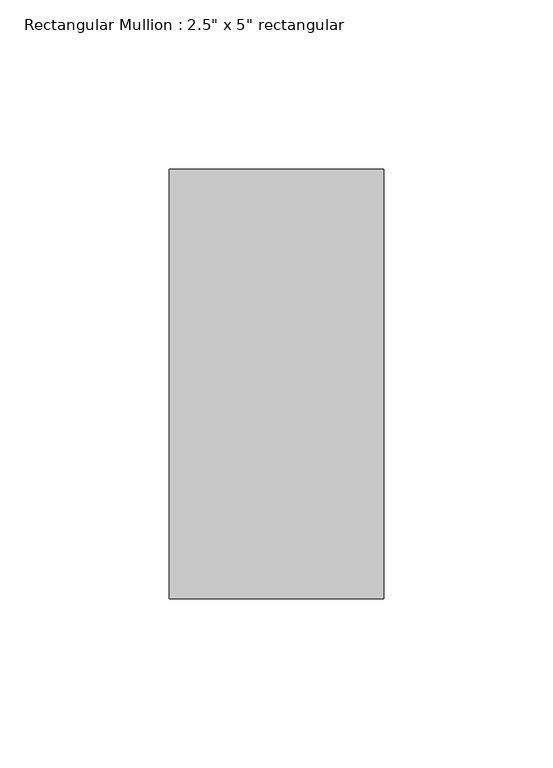
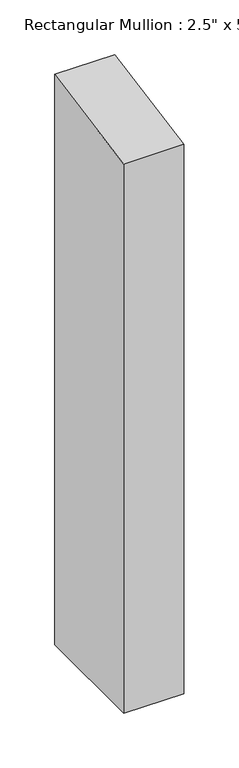
"""IFC4 building model written with IfcOpenShell, lengths in millimetres: member geometry."""

from ifc_helpers import new_model, si_unit, frame, origin, place, context, project, spatial, polyline, outline, extrude, source, transform, mapped, element, save


def member_73d0c9ee(model_context):
    return source(origin(), model_context, "Body", "SweptSolid", [
        extrude(outline(polyline([(-63.5, -11.6039351), (63.5, 11.6039351), (63.5, -625.8413472), (-63.5, -625.8413472), (-63.5, -11.6039351)])), frame((-63.5, 0.0, 0.0), z_axis=(1.0, 0.0, 0.0), x_axis=(0.0, 1.0, 0.0)), (0.0, 0.0, 1.0), 63.5),
    ])


if __name__ == "__main__":
    model = new_model("IFC4")
    model_context = context("Model", 3, world=origin())
    ifc_project = project(units=[si_unit("LENGTHUNIT", "METRE", prefix="MILLI")], contexts=[model_context])
    site = spatial("IfcSite", under=ifc_project)
    building = spatial("IfcBuilding", under=site)
    placement = place(None, origin())
    member_shape = member_73d0c9ee(model_context)
    element("IfcMember", 1, ObjectType="Rectangular Mullion : 2.5\" x 5\" rectangular", at=placement, inside=building, context=model_context, shape_type="MappedRepresentation", body=[
        mapped(member_shape, transform((0.0, 0.0, 0.0), x_axis=(1.0, 0.0, 0.0), y_axis=(0.0, 1.0, 0.0), z_axis=(0.0, 0.0, 1.0))),
    ])
    save(model, "model.ifc")

# Revit data of these elements
# Type "Rectangular Mullion : 2.5\" x 5\" rectangular"
#   built-in parameter 1007304 = 0.416667 (stored number, unit not read)
#   built-in parameter 1007301 = 0.104167 (stored number, unit not read)
#   built-in parameter 1007300 = 0.104167 (stored number, unit not read)
# Element 1 (IfcMember, "Rectangular Mullion : 2.5\" x 5\" rectangular")
#   Materials on its faces: "Iron, Ductile"
# Materials
#   "Iron, Ductile": class "Metal", colour RGB 0 0 0, transparency 0, Description = "Ductile cast iron", Cost = 0
